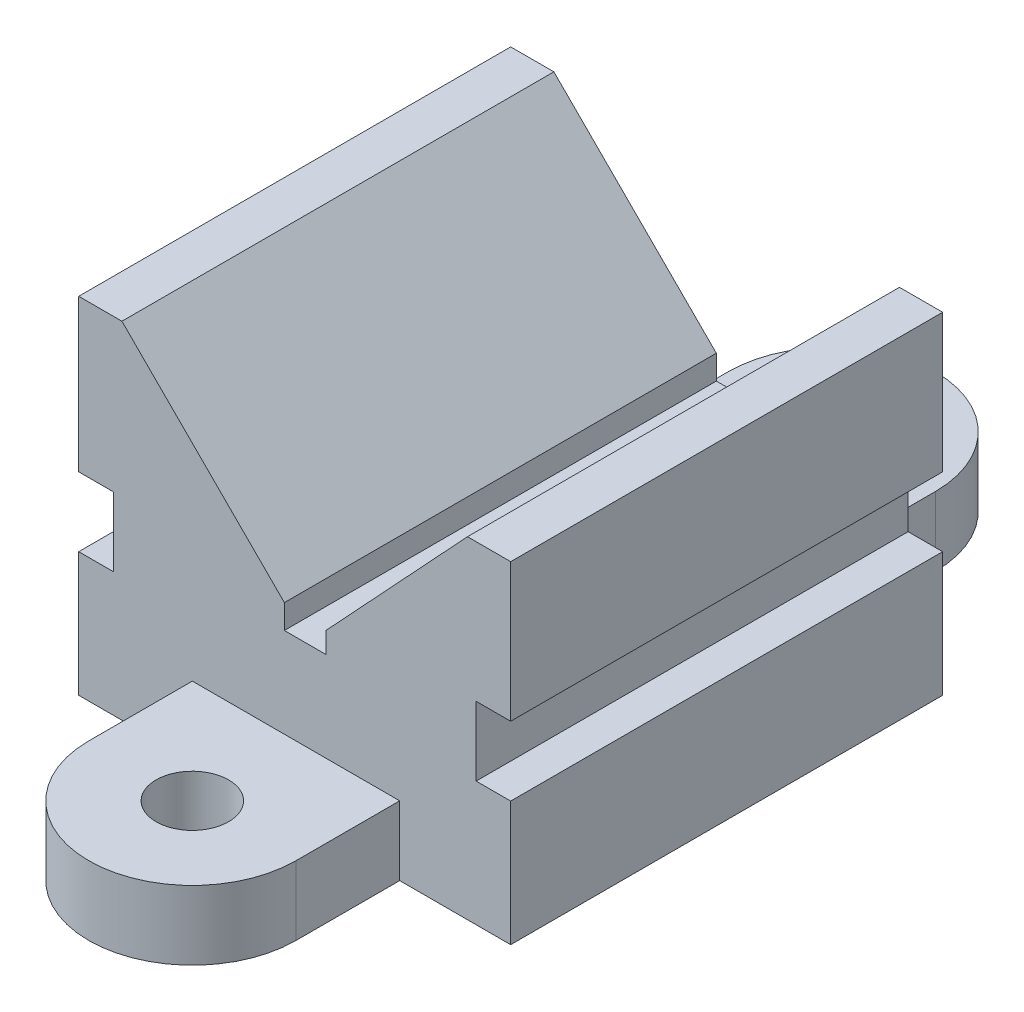
ISO-10303-21;
HEADER;
FILE_DESCRIPTION(('STEP AP214'),'2;1');
FILE_NAME('part.step','',(''),(''),'','','');
FILE_SCHEMA(('AUTOMOTIVE_DESIGN { 1 0 10303 214 1 1 1 1 }'));
ENDSEC;
DATA;
#1=APPLICATION_CONTEXT('core data for automotive mechanical design processes');
#2=APPLICATION_PROTOCOL_DEFINITION('international standard','automotive_design',2000,#1);
#3=PRODUCT_CONTEXT('',#1,'mechanical');
#4=PRODUCT('Part','Part','',(#3));
#5=PRODUCT_RELATED_PRODUCT_CATEGORY('part','',(#4));
#6=PRODUCT_DEFINITION_FORMATION('','',#4);
#7=PRODUCT_DEFINITION_CONTEXT('part definition',#1,'design');
#8=PRODUCT_DEFINITION('design','',#6,#7);
#9=PRODUCT_DEFINITION_SHAPE('','',#8);
#10=(LENGTH_UNIT() NAMED_UNIT(*) SI_UNIT(.MILLI.,.METRE.));
#11=(NAMED_UNIT(*) PLANE_ANGLE_UNIT() SI_UNIT($,.RADIAN.));
#12=(NAMED_UNIT(*) SI_UNIT($,.STERADIAN.) SOLID_ANGLE_UNIT());
#13=UNCERTAINTY_MEASURE_WITH_UNIT(LENGTH_MEASURE(1.E-05),#10,'distance_accuracy_value','');
#14=(GEOMETRIC_REPRESENTATION_CONTEXT(3) GLOBAL_UNCERTAINTY_ASSIGNED_CONTEXT((#13)) GLOBAL_UNIT_ASSIGNED_CONTEXT((#10,
#11,#12)) REPRESENTATION_CONTEXT('',''));
#15=CARTESIAN_POINT('',(0.,0.,0.));
#16=DIRECTION('',(0.,0.,1.));
#17=DIRECTION('',(1.,0.,0.));
#18=AXIS2_PLACEMENT_3D('',#15,#16,#17);
#19=CARTESIAN_POINT('',(-40.4580152671756,36.,125.));
#20=DIRECTION('',(1.,0.,0.));
#21=DIRECTION('',(0.,1.,0.));
#22=AXIS2_PLACEMENT_3D('',#19,#20,#21);
#23=PLANE('',#22);
#24=DIRECTION('',(0.,-1.,0.));
#25=VECTOR('',#24,1.);
#26=CARTESIAN_POINT('',(-40.4580152671756,36.,0.));
#27=LINE('',#26,#25);
#28=CARTESIAN_POINT('',(-40.4580152671756,36.,0.));
#29=VERTEX_POINT('',#28);
#30=CARTESIAN_POINT('',(-40.4580152671756,0.,0.));
#31=VERTEX_POINT('',#30);
#32=EDGE_CURVE('E266',#29,#31,#27,.T.);
#33=ORIENTED_EDGE('',*,*,#32,.T.);
#34=DIRECTION('',(0.,0.,-1.));
#35=VECTOR('',#34,1.);
#36=CARTESIAN_POINT('',(-40.4580152671756,0.,125.));
#37=LINE('',#36,#35);
#38=CARTESIAN_POINT('',(-40.4580152671756,0.,125.));
#39=VERTEX_POINT('',#38);
#40=EDGE_CURVE('E393',#39,#31,#37,.T.);
#41=ORIENTED_EDGE('',*,*,#40,.F.);
#42=DIRECTION('',(0.,-1.,0.));
#43=VECTOR('',#42,1.);
#44=CARTESIAN_POINT('',(-40.4580152671756,36.,125.));
#45=LINE('',#44,#43);
#46=CARTESIAN_POINT('',(-40.4580152671756,36.,125.));
#47=VERTEX_POINT('',#46);
#48=EDGE_CURVE('E270',#47,#39,#45,.T.);
#49=ORIENTED_EDGE('',*,*,#48,.F.);
#50=DIRECTION('',(0.,0.,-1.));
#51=VECTOR('',#50,1.);
#52=CARTESIAN_POINT('',(-40.4580152671756,36.,125.));
#53=LINE('',#52,#51);
#54=EDGE_CURVE('E308',#47,#29,#53,.T.);
#55=ORIENTED_EDGE('',*,*,#54,.T.);
#56=EDGE_LOOP('',(#33,#41,#49,#55));
#57=FACE_BOUND('',#56,.T.);
#58=ADVANCED_FACE('F39',(#57),#23,.F.);
#59=CARTESIAN_POINT('',(-40.4580152671756,0.,125.));
#60=DIRECTION('',(0.,1.,0.));
#61=DIRECTION('',(0.,0.,1.));
#62=AXIS2_PLACEMENT_3D('',#59,#60,#61);
#63=PLANE('',#62);
#64=DIRECTION('',(1.,0.,0.));
#65=VECTOR('',#64,1.);
#66=CARTESIAN_POINT('',(-40.4580152671756,0.,0.));
#67=LINE('',#66,#65);
#68=CARTESIAN_POINT('',(-7.57863831219291,0.,0.));
#69=VERTEX_POINT('',#68);
#70=EDGE_CURVE('E309',#31,#69,#67,.T.);
#71=ORIENTED_EDGE('',*,*,#70,.T.);
#72=DIRECTION('',(0.,0.,-1.));
#73=VECTOR('',#72,1.);
#74=CARTESIAN_POINT('',(-7.57863831219292,0.,155.));
#75=LINE('',#74,#73);
#76=CARTESIAN_POINT('',(-7.5786383121929,0.,-30.));
#77=VERTEX_POINT('',#76);
#78=EDGE_CURVE('E253',#69,#77,#75,.T.);
#79=ORIENTED_EDGE('',*,*,#78,.T.);
#80=CARTESIAN_POINT('',(22.4213616878071,0.,-30.));
#81=DIRECTION('',(0.,-1.,0.));
#82=DIRECTION('',(0.,0.,-1.));
#83=AXIS2_PLACEMENT_3D('',#80,#81,#82);
#84=CIRCLE('',#83,30.);
#85=CARTESIAN_POINT('',(52.4213616878071,0.,-30.));
#86=VERTEX_POINT('',#85);
#87=EDGE_CURVE('E255',#77,#86,#84,.T.);
#88=ORIENTED_EDGE('',*,*,#87,.T.);
#89=DIRECTION('',(0.,0.,1.));
#90=VECTOR('',#89,1.);
#91=CARTESIAN_POINT('',(52.4213616878071,0.,155.));
#92=LINE('',#91,#90);
#93=CARTESIAN_POINT('',(52.4213616878071,0.,0.));
#94=VERTEX_POINT('',#93);
#95=EDGE_CURVE('E237',#86,#94,#92,.T.);
#96=ORIENTED_EDGE('',*,*,#95,.T.);
#97=CARTESIAN_POINT('',(84.5419847328244,0.,0.));
#98=VERTEX_POINT('',#97);
#99=EDGE_CURVE('E310',#94,#98,#67,.T.);
#100=ORIENTED_EDGE('',*,*,#99,.T.);
#101=DIRECTION('',(0.,0.,-1.));
#102=VECTOR('',#101,1.);
#103=CARTESIAN_POINT('',(84.5419847328244,0.,125.));
#104=LINE('',#103,#102);
#105=CARTESIAN_POINT('',(84.5419847328244,0.,125.));
#106=VERTEX_POINT('',#105);
#107=EDGE_CURVE('E391',#106,#98,#104,.T.);
#108=ORIENTED_EDGE('',*,*,#107,.F.);
#109=DIRECTION('',(1.,0.,0.));
#110=VECTOR('',#109,1.);
#111=CARTESIAN_POINT('',(-40.4580152671756,0.,125.));
#112=LINE('',#111,#110);
#113=CARTESIAN_POINT('',(52.4213616878071,0.,125.));
#114=VERTEX_POINT('',#113);
#115=EDGE_CURVE('E269',#114,#106,#112,.T.);
#116=ORIENTED_EDGE('',*,*,#115,.F.);
#117=CARTESIAN_POINT('',(52.4213616878071,0.,155.));
#118=VERTEX_POINT('',#117);
#119=EDGE_CURVE('E236',#114,#118,#92,.T.);
#120=ORIENTED_EDGE('',*,*,#119,.T.);
#121=CARTESIAN_POINT('',(22.4213616878071,0.,155.));
#122=DIRECTION('',(0.,-1.,0.));
#123=DIRECTION('',(0.,0.,-1.));
#124=AXIS2_PLACEMENT_3D('',#121,#122,#123);
#125=CIRCLE('',#124,30.);
#126=CARTESIAN_POINT('',(-7.57863831219292,0.,155.));
#127=VERTEX_POINT('',#126);
#128=EDGE_CURVE('E248',#118,#127,#125,.T.);
#129=ORIENTED_EDGE('',*,*,#128,.T.);
#130=CARTESIAN_POINT('',(-7.57863831219293,0.,125.));
#131=VERTEX_POINT('',#130);
#132=EDGE_CURVE('E214',#127,#131,#75,.T.);
#133=ORIENTED_EDGE('',*,*,#132,.T.);
#134=EDGE_CURVE('E275',#39,#131,#112,.T.);
#135=ORIENTED_EDGE('',*,*,#134,.F.);
#136=ORIENTED_EDGE('',*,*,#40,.T.);
#137=EDGE_LOOP('',(#71,#79,#88,#96,#100,#108,#116,#120,#129,#133,#135,#136));
#138=FACE_BOUND('',#137,.T.);
#139=CARTESIAN_POINT('',(22.4213616878071,0.,-30.));
#140=DIRECTION('',(0.,-1.,0.));
#141=DIRECTION('',(0.,0.,-1.));
#142=AXIS2_PLACEMENT_3D('',#139,#140,#141);
#143=CIRCLE('',#142,10.5);
#144=CARTESIAN_POINT('',(22.4213616878071,0.,-40.5));
#145=VERTEX_POINT('',#144);
#146=EDGE_CURVE('E241',#145,#145,#143,.T.);
#147=ORIENTED_EDGE('',*,*,#146,.F.);
#148=EDGE_LOOP('',(#147));
#149=FACE_BOUND('',#148,.T.);
#150=CARTESIAN_POINT('',(22.4213616878071,0.,155.));
#151=DIRECTION('',(0.,-1.,0.));
#152=DIRECTION('',(0.,0.,-1.));
#153=AXIS2_PLACEMENT_3D('',#150,#151,#152);
#154=CIRCLE('',#153,10.5);
#155=CARTESIAN_POINT('',(22.4213616878071,0.,144.5));
#156=VERTEX_POINT('',#155);
#157=EDGE_CURVE('E587',#156,#156,#154,.T.);
#158=ORIENTED_EDGE('',*,*,#157,.F.);
#159=EDGE_LOOP('',(#158));
#160=FACE_BOUND('',#159,.T.);
#161=ADVANCED_FACE('F410',(#138,#149,#160),#63,.F.);
#162=CARTESIAN_POINT('',(84.5419847328244,0.,125.));
#163=DIRECTION('',(-1.,0.,0.));
#164=DIRECTION('',(0.,-1.,0.));
#165=AXIS2_PLACEMENT_3D('',#162,#163,#164);
#166=PLANE('',#165);
#167=DIRECTION('',(0.,1.,0.));
#168=VECTOR('',#167,1.);
#169=CARTESIAN_POINT('',(84.5419847328244,0.,0.));
#170=LINE('',#169,#168);
#171=CARTESIAN_POINT('',(84.5419847328244,36.,0.));
#172=VERTEX_POINT('',#171);
#173=EDGE_CURVE('E311',#98,#172,#170,.T.);
#174=ORIENTED_EDGE('',*,*,#173,.T.);
#175=DIRECTION('',(0.,0.,-1.));
#176=VECTOR('',#175,1.);
#177=CARTESIAN_POINT('',(84.5419847328244,36.,125.));
#178=LINE('',#177,#176);
#179=CARTESIAN_POINT('',(84.5419847328244,36.,125.));
#180=VERTEX_POINT('',#179);
#181=EDGE_CURVE('E389',#180,#172,#178,.T.);
#182=ORIENTED_EDGE('',*,*,#181,.F.);
#183=DIRECTION('',(0.,1.,0.));
#184=VECTOR('',#183,1.);
#185=CARTESIAN_POINT('',(84.5419847328244,0.,125.));
#186=LINE('',#185,#184);
#187=EDGE_CURVE('E273',#106,#180,#186,.T.);
#188=ORIENTED_EDGE('',*,*,#187,.F.);
#189=ORIENTED_EDGE('',*,*,#107,.T.);
#190=EDGE_LOOP('',(#174,#182,#188,#189));
#191=FACE_BOUND('',#190,.T.);
#192=ADVANCED_FACE('F489',(#191),#166,.F.);
#193=CARTESIAN_POINT('',(84.5419847328244,36.,125.));
#194=DIRECTION('',(0.,-1.,0.));
#195=DIRECTION('',(1.,0.,0.));
#196=AXIS2_PLACEMENT_3D('',#193,#194,#195);
#197=PLANE('',#196);
#198=DIRECTION('',(-1.,0.,0.));
#199=VECTOR('',#198,1.);
#200=CARTESIAN_POINT('',(84.5419847328244,36.,0.));
#201=LINE('',#200,#199);
#202=CARTESIAN_POINT('',(74.5419847328244,36.,0.));
#203=VERTEX_POINT('',#202);
#204=EDGE_CURVE('E312',#172,#203,#201,.T.);
#205=ORIENTED_EDGE('',*,*,#204,.T.);
#206=DIRECTION('',(0.,0.,-1.));
#207=VECTOR('',#206,1.);
#208=CARTESIAN_POINT('',(74.5419847328244,36.,125.));
#209=LINE('',#208,#207);
#210=CARTESIAN_POINT('',(74.5419847328244,36.,125.));
#211=VERTEX_POINT('',#210);
#212=EDGE_CURVE('E384',#211,#203,#209,.T.);
#213=ORIENTED_EDGE('',*,*,#212,.F.);
#214=DIRECTION('',(-1.,0.,0.));
#215=VECTOR('',#214,1.);
#216=CARTESIAN_POINT('',(84.5419847328244,36.,125.));
#217=LINE('',#216,#215);
#218=EDGE_CURVE('E277',#180,#211,#217,.T.);
#219=ORIENTED_EDGE('',*,*,#218,.F.);
#220=ORIENTED_EDGE('',*,*,#181,.T.);
#221=EDGE_LOOP('',(#205,#213,#219,#220));
#222=FACE_BOUND('',#221,.T.);
#223=ADVANCED_FACE('F486',(#222),#197,.F.);
#224=CARTESIAN_POINT('',(74.5419847328244,36.,125.));
#225=DIRECTION('',(-1.,0.,0.));
#226=DIRECTION('',(0.,0.,1.));
#227=AXIS2_PLACEMENT_3D('',#224,#225,#226);
#228=PLANE('',#227);
#229=DIRECTION('',(0.,1.,0.));
#230=VECTOR('',#229,1.);
#231=CARTESIAN_POINT('',(74.5419847328244,36.,0.));
#232=LINE('',#231,#230);
#233=CARTESIAN_POINT('',(74.5419847328244,56.,0.));
#234=VERTEX_POINT('',#233);
#235=EDGE_CURVE('E320',#203,#234,#232,.T.);
#236=ORIENTED_EDGE('',*,*,#235,.T.);
#237=DIRECTION('',(0.,0.,-1.));
#238=VECTOR('',#237,1.);
#239=CARTESIAN_POINT('',(74.5419847328244,56.,125.));
#240=LINE('',#239,#238);
#241=CARTESIAN_POINT('',(74.5419847328244,56.,125.));
#242=VERTEX_POINT('',#241);
#243=EDGE_CURVE('E385',#242,#234,#240,.T.);
#244=ORIENTED_EDGE('',*,*,#243,.F.);
#245=DIRECTION('',(0.,1.,0.));
#246=VECTOR('',#245,1.);
#247=CARTESIAN_POINT('',(74.5419847328244,36.,125.));
#248=LINE('',#247,#246);
#249=EDGE_CURVE('E279',#211,#242,#248,.T.);
#250=ORIENTED_EDGE('',*,*,#249,.F.);
#251=ORIENTED_EDGE('',*,*,#212,.T.);
#252=EDGE_LOOP('',(#236,#244,#250,#251));
#253=FACE_BOUND('',#252,.T.);
#254=ADVANCED_FACE('F485',(#253),#228,.F.);
#255=CARTESIAN_POINT('',(74.5419847328244,56.,125.));
#256=DIRECTION('',(0.,1.,0.));
#257=DIRECTION('',(0.,0.,1.));
#258=AXIS2_PLACEMENT_3D('',#255,#256,#257);
#259=PLANE('',#258);
#260=DIRECTION('',(1.,0.,0.));
#261=VECTOR('',#260,1.);
#262=CARTESIAN_POINT('',(74.5419847328244,56.,0.));
#263=LINE('',#262,#261);
#264=CARTESIAN_POINT('',(84.5419847328244,56.,0.));
#265=VERTEX_POINT('',#264);
#266=EDGE_CURVE('E317',#234,#265,#263,.T.);
#267=ORIENTED_EDGE('',*,*,#266,.T.);
#268=DIRECTION('',(0.,0.,-1.));
#269=VECTOR('',#268,1.);
#270=CARTESIAN_POINT('',(84.5419847328244,56.,125.));
#271=LINE('',#270,#269);
#272=CARTESIAN_POINT('',(84.5419847328244,56.,125.));
#273=VERTEX_POINT('',#272);
#274=EDGE_CURVE('E377',#273,#265,#271,.T.);
#275=ORIENTED_EDGE('',*,*,#274,.F.);
#276=DIRECTION('',(1.,0.,0.));
#277=VECTOR('',#276,1.);
#278=CARTESIAN_POINT('',(74.5419847328244,56.,125.));
#279=LINE('',#278,#277);
#280=EDGE_CURVE('E278',#242,#273,#279,.T.);
#281=ORIENTED_EDGE('',*,*,#280,.F.);
#282=ORIENTED_EDGE('',*,*,#243,.T.);
#283=EDGE_LOOP('',(#267,#275,#281,#282));
#284=FACE_BOUND('',#283,.T.);
#285=ADVANCED_FACE('F480',(#284),#259,.F.);
#286=CARTESIAN_POINT('',(84.5419847328244,56.,125.));
#287=DIRECTION('',(-1.,0.,0.));
#288=DIRECTION('',(0.,0.,1.));
#289=AXIS2_PLACEMENT_3D('',#286,#287,#288);
#290=PLANE('',#289);
#291=DIRECTION('',(0.,1.,0.));
#292=VECTOR('',#291,1.);
#293=CARTESIAN_POINT('',(84.5419847328244,56.,0.));
#294=LINE('',#293,#292);
#295=CARTESIAN_POINT('',(84.5419847328244,96.,0.));
#296=VERTEX_POINT('',#295);
#297=EDGE_CURVE('E321',#265,#296,#294,.T.);
#298=ORIENTED_EDGE('',*,*,#297,.T.);
#299=DIRECTION('',(0.,0.,-1.));
#300=VECTOR('',#299,1.);
#301=CARTESIAN_POINT('',(84.5419847328244,96.,125.));
#302=LINE('',#301,#300);
#303=CARTESIAN_POINT('',(84.5419847328244,96.,125.));
#304=VERTEX_POINT('',#303);
#305=EDGE_CURVE('E376',#304,#296,#302,.T.);
#306=ORIENTED_EDGE('',*,*,#305,.F.);
#307=DIRECTION('',(0.,1.,0.));
#308=VECTOR('',#307,1.);
#309=CARTESIAN_POINT('',(84.5419847328244,56.,125.));
#310=LINE('',#309,#308);
#311=EDGE_CURVE('E285',#273,#304,#310,.T.);
#312=ORIENTED_EDGE('',*,*,#311,.F.);
#313=ORIENTED_EDGE('',*,*,#274,.T.);
#314=EDGE_LOOP('',(#298,#306,#312,#313));
#315=FACE_BOUND('',#314,.T.);
#316=ADVANCED_FACE('F473',(#315),#290,.F.);
#317=CARTESIAN_POINT('',(84.5419847328244,96.,125.));
#318=DIRECTION('',(0.,-1.,0.));
#319=DIRECTION('',(0.,0.,-1.));
#320=AXIS2_PLACEMENT_3D('',#317,#318,#319);
#321=PLANE('',#320);
#322=DIRECTION('',(-1.,0.,0.));
#323=VECTOR('',#322,1.);
#324=CARTESIAN_POINT('',(84.5419847328244,96.,0.));
#325=LINE('',#324,#323);
#326=CARTESIAN_POINT('',(72.0419847328244,96.,0.));
#327=VERTEX_POINT('',#326);
#328=EDGE_CURVE('E323',#296,#327,#325,.T.);
#329=ORIENTED_EDGE('',*,*,#328,.T.);
#330=DIRECTION('',(0.,0.,-1.));
#331=VECTOR('',#330,1.);
#332=CARTESIAN_POINT('',(72.0419847328244,96.,125.));
#333=LINE('',#332,#331);
#334=CARTESIAN_POINT('',(72.0419847328244,96.,125.));
#335=VERTEX_POINT('',#334);
#336=EDGE_CURVE('E373',#335,#327,#333,.T.);
#337=ORIENTED_EDGE('',*,*,#336,.F.);
#338=DIRECTION('',(-1.,0.,0.));
#339=VECTOR('',#338,1.);
#340=CARTESIAN_POINT('',(84.5419847328244,96.,125.));
#341=LINE('',#340,#339);
#342=EDGE_CURVE('E283',#304,#335,#341,.T.);
#343=ORIENTED_EDGE('',*,*,#342,.F.);
#344=ORIENTED_EDGE('',*,*,#305,.T.);
#345=EDGE_LOOP('',(#329,#337,#343,#344));
#346=FACE_BOUND('',#345,.T.);
#347=ADVANCED_FACE('F470',(#346),#321,.F.);
#348=CARTESIAN_POINT('',(72.0419847328244,96.,125.));
#349=DIRECTION('',(0.731695452994903,-0.68163169238716,0.));
#350=DIRECTION('',(0.68163169238716,0.731695452994903,0.));
#351=AXIS2_PLACEMENT_3D('',#348,#349,#350);
#352=PLANE('',#351);
#353=DIRECTION('',(-0.68163169238716,-0.731695452994903,0.));
#354=VECTOR('',#353,1.);
#355=CARTESIAN_POINT('',(72.0419847328244,96.,0.));
#356=LINE('',#355,#354);
#357=CARTESIAN_POINT('',(31.052534351145,52.,0.));
#358=VERTEX_POINT('',#357);
#359=EDGE_CURVE('E324',#327,#358,#356,.T.);
#360=ORIENTED_EDGE('',*,*,#359,.T.);
#361=DIRECTION('',(0.,0.,-1.));
#362=VECTOR('',#361,1.);
#363=CARTESIAN_POINT('',(31.052534351145,52.,125.));
#364=LINE('',#363,#362);
#365=CARTESIAN_POINT('',(31.052534351145,52.,125.));
#366=VERTEX_POINT('',#365);
#367=EDGE_CURVE('E367',#366,#358,#364,.T.);
#368=ORIENTED_EDGE('',*,*,#367,.F.);
#369=DIRECTION('',(-0.68163169238716,-0.731695452994903,0.));
#370=VECTOR('',#369,1.);
#371=CARTESIAN_POINT('',(72.0419847328244,96.,125.));
#372=LINE('',#371,#370);
#373=EDGE_CURVE('E286',#335,#366,#372,.T.);
#374=ORIENTED_EDGE('',*,*,#373,.F.);
#375=ORIENTED_EDGE('',*,*,#336,.T.);
#376=EDGE_LOOP('',(#360,#368,#374,#375));
#377=FACE_BOUND('',#376,.T.);
#378=ADVANCED_FACE('F465',(#377),#352,.F.);
#379=CARTESIAN_POINT('',(31.052534351145,52.,125.));
#380=DIRECTION('',(1.,0.,0.));
#381=DIRECTION('',(0.,1.,0.));
#382=AXIS2_PLACEMENT_3D('',#379,#380,#381);
#383=PLANE('',#382);
#384=DIRECTION('',(0.,-1.,0.));
#385=VECTOR('',#384,1.);
#386=CARTESIAN_POINT('',(31.052534351145,52.,0.));
#387=LINE('',#386,#385);
#388=CARTESIAN_POINT('',(31.052534351145,46.,0.));
#389=VERTEX_POINT('',#388);
#390=EDGE_CURVE('E330',#358,#389,#387,.T.);
#391=ORIENTED_EDGE('',*,*,#390,.T.);
#392=DIRECTION('',(0.,0.,-1.));
#393=VECTOR('',#392,1.);
#394=CARTESIAN_POINT('',(31.052534351145,46.,125.));
#395=LINE('',#394,#393);
#396=CARTESIAN_POINT('',(31.052534351145,46.,125.));
#397=VERTEX_POINT('',#396);
#398=EDGE_CURVE('E370',#397,#389,#395,.T.);
#399=ORIENTED_EDGE('',*,*,#398,.F.);
#400=DIRECTION('',(0.,-1.,0.));
#401=VECTOR('',#400,1.);
#402=CARTESIAN_POINT('',(31.052534351145,52.,125.));
#403=LINE('',#402,#401);
#404=EDGE_CURVE('E287',#366,#397,#403,.T.);
#405=ORIENTED_EDGE('',*,*,#404,.F.);
#406=ORIENTED_EDGE('',*,*,#367,.T.);
#407=EDGE_LOOP('',(#391,#399,#405,#406));
#408=FACE_BOUND('',#407,.T.);
#409=ADVANCED_FACE('F457',(#408),#383,.F.);
#410=CARTESIAN_POINT('',(31.052534351145,46.,125.));
#411=DIRECTION('',(0.,-1.,0.));
#412=DIRECTION('',(1.,0.,0.));
#413=AXIS2_PLACEMENT_3D('',#410,#411,#412);
#414=PLANE('',#413);
#415=DIRECTION('',(-1.,0.,0.));
#416=VECTOR('',#415,1.);
#417=CARTESIAN_POINT('',(31.052534351145,46.,0.));
#418=LINE('',#417,#416);
#419=CARTESIAN_POINT('',(19.052534351145,46.,0.));
#420=VERTEX_POINT('',#419);
#421=EDGE_CURVE('E328',#389,#420,#418,.T.);
#422=ORIENTED_EDGE('',*,*,#421,.T.);
#423=DIRECTION('',(0.,0.,-1.));
#424=VECTOR('',#423,1.);
#425=CARTESIAN_POINT('',(19.052534351145,46.,125.));
#426=LINE('',#425,#424);
#427=CARTESIAN_POINT('',(19.052534351145,46.,125.));
#428=VERTEX_POINT('',#427);
#429=EDGE_CURVE('E365',#428,#420,#426,.T.);
#430=ORIENTED_EDGE('',*,*,#429,.F.);
#431=DIRECTION('',(-1.,0.,0.));
#432=VECTOR('',#431,1.);
#433=CARTESIAN_POINT('',(31.052534351145,46.,125.));
#434=LINE('',#433,#432);
#435=EDGE_CURVE('E289',#397,#428,#434,.T.);
#436=ORIENTED_EDGE('',*,*,#435,.F.);
#437=ORIENTED_EDGE('',*,*,#398,.T.);
#438=EDGE_LOOP('',(#422,#430,#436,#437));
#439=FACE_BOUND('',#438,.T.);
#440=ADVANCED_FACE('F455',(#439),#414,.F.);
#441=CARTESIAN_POINT('',(19.052534351145,46.,125.));
#442=DIRECTION('',(-1.,0.,0.));
#443=DIRECTION('',(0.,-1.,0.));
#444=AXIS2_PLACEMENT_3D('',#441,#442,#443);
#445=PLANE('',#444);
#446=DIRECTION('',(0.,1.,0.));
#447=VECTOR('',#446,1.);
#448=CARTESIAN_POINT('',(19.052534351145,46.,0.));
#449=LINE('',#448,#447);
#450=CARTESIAN_POINT('',(19.052534351145,52.9894503816794,0.));
#451=VERTEX_POINT('',#450);
#452=EDGE_CURVE('E332',#420,#451,#449,.T.);
#453=ORIENTED_EDGE('',*,*,#452,.T.);
#454=DIRECTION('',(0.,0.,-1.));
#455=VECTOR('',#454,1.);
#456=CARTESIAN_POINT('',(19.052534351145,52.9894503816794,125.));
#457=LINE('',#456,#455);
#458=CARTESIAN_POINT('',(19.052534351145,52.9894503816794,125.));
#459=VERTEX_POINT('',#458);
#460=EDGE_CURVE('E363',#459,#451,#457,.T.);
#461=ORIENTED_EDGE('',*,*,#460,.F.);
#462=DIRECTION('',(0.,1.,0.));
#463=VECTOR('',#462,1.);
#464=CARTESIAN_POINT('',(19.052534351145,46.,125.));
#465=LINE('',#464,#463);
#466=EDGE_CURVE('E295',#428,#459,#465,.T.);
#467=ORIENTED_EDGE('',*,*,#466,.F.);
#468=ORIENTED_EDGE('',*,*,#429,.T.);
#469=EDGE_LOOP('',(#453,#461,#467,#468));
#470=FACE_BOUND('',#469,.T.);
#471=ADVANCED_FACE('F450',(#470),#445,.F.);
#472=CARTESIAN_POINT('',(19.052534351145,52.9894503816794,125.));
#473=DIRECTION('',(-0.707106781186547,-0.707106781186548,0.));
#474=DIRECTION('',(0.707106781186548,-0.707106781186547,0.));
#475=AXIS2_PLACEMENT_3D('',#472,#473,#474);
#476=PLANE('',#475);
#477=DIRECTION('',(-0.707106781186548,0.707106781186547,0.));
#478=VECTOR('',#477,1.);
#479=CARTESIAN_POINT('',(19.052534351145,52.9894503816794,0.));
#480=LINE('',#479,#478);
#481=CARTESIAN_POINT('',(-27.9580152671756,100.,0.));
#482=VERTEX_POINT('',#481);
#483=EDGE_CURVE('E334',#451,#482,#480,.T.);
#484=ORIENTED_EDGE('',*,*,#483,.T.);
#485=DIRECTION('',(0.,0.,-1.));
#486=VECTOR('',#485,1.);
#487=CARTESIAN_POINT('',(-27.9580152671756,100.,125.));
#488=LINE('',#487,#486);
#489=CARTESIAN_POINT('',(-27.9580152671756,100.,125.));
#490=VERTEX_POINT('',#489);
#491=EDGE_CURVE('E357',#490,#482,#488,.T.);
#492=ORIENTED_EDGE('',*,*,#491,.F.);
#493=DIRECTION('',(-0.707106781186548,0.707106781186547,0.));
#494=VECTOR('',#493,1.);
#495=CARTESIAN_POINT('',(19.052534351145,52.9894503816794,125.));
#496=LINE('',#495,#494);
#497=EDGE_CURVE('E294',#459,#490,#496,.T.);
#498=ORIENTED_EDGE('',*,*,#497,.F.);
#499=ORIENTED_EDGE('',*,*,#460,.T.);
#500=EDGE_LOOP('',(#484,#492,#498,#499));
#501=FACE_BOUND('',#500,.T.);
#502=ADVANCED_FACE('F442',(#501),#476,.F.);
#503=CARTESIAN_POINT('',(-27.9580152671756,100.,125.));
#504=DIRECTION('',(0.,-1.,0.));
#505=DIRECTION('',(0.,0.,-1.));
#506=AXIS2_PLACEMENT_3D('',#503,#504,#505);
#507=PLANE('',#506);
#508=DIRECTION('',(-1.,0.,0.));
#509=VECTOR('',#508,1.);
#510=CARTESIAN_POINT('',(-27.9580152671756,100.,0.));
#511=LINE('',#510,#509);
#512=CARTESIAN_POINT('',(-40.4580152671756,100.,0.));
#513=VERTEX_POINT('',#512);
#514=EDGE_CURVE('E333',#482,#513,#511,.T.);
#515=ORIENTED_EDGE('',*,*,#514,.T.);
#516=DIRECTION('',(0.,0.,-1.));
#517=VECTOR('',#516,1.);
#518=CARTESIAN_POINT('',(-40.4580152671756,100.,125.));
#519=LINE('',#518,#517);
#520=CARTESIAN_POINT('',(-40.4580152671756,100.,125.));
#521=VERTEX_POINT('',#520);
#522=EDGE_CURVE('E354',#521,#513,#519,.T.);
#523=ORIENTED_EDGE('',*,*,#522,.F.);
#524=DIRECTION('',(-1.,0.,0.));
#525=VECTOR('',#524,1.);
#526=CARTESIAN_POINT('',(-27.9580152671756,100.,125.));
#527=LINE('',#526,#525);
#528=EDGE_CURVE('E296',#490,#521,#527,.T.);
#529=ORIENTED_EDGE('',*,*,#528,.F.);
#530=ORIENTED_EDGE('',*,*,#491,.T.);
#531=EDGE_LOOP('',(#515,#523,#529,#530));
#532=FACE_BOUND('',#531,.T.);
#533=ADVANCED_FACE('F440',(#532),#507,.F.);
#534=CARTESIAN_POINT('',(-40.4580152671756,100.,125.));
#535=DIRECTION('',(1.,0.,0.));
#536=DIRECTION('',(0.,1.,0.));
#537=AXIS2_PLACEMENT_3D('',#534,#535,#536);
#538=PLANE('',#537);
#539=DIRECTION('',(0.,-1.,0.));
#540=VECTOR('',#539,1.);
#541=CARTESIAN_POINT('',(-40.4580152671756,100.,0.));
#542=LINE('',#541,#540);
#543=CARTESIAN_POINT('',(-40.4580152671756,56.,0.));
#544=VERTEX_POINT('',#543);
#545=EDGE_CURVE('E340',#513,#544,#542,.T.);
#546=ORIENTED_EDGE('',*,*,#545,.T.);
#547=DIRECTION('',(0.,0.,-1.));
#548=VECTOR('',#547,1.);
#549=CARTESIAN_POINT('',(-40.4580152671756,56.,125.));
#550=LINE('',#549,#548);
#551=CARTESIAN_POINT('',(-40.4580152671756,56.,125.));
#552=VERTEX_POINT('',#551);
#553=EDGE_CURVE('E355',#552,#544,#550,.T.);
#554=ORIENTED_EDGE('',*,*,#553,.F.);
#555=DIRECTION('',(0.,-1.,0.));
#556=VECTOR('',#555,1.);
#557=CARTESIAN_POINT('',(-40.4580152671756,100.,125.));
#558=LINE('',#557,#556);
#559=EDGE_CURVE('E297',#521,#552,#558,.T.);
#560=ORIENTED_EDGE('',*,*,#559,.F.);
#561=ORIENTED_EDGE('',*,*,#522,.T.);
#562=EDGE_LOOP('',(#546,#554,#560,#561));
#563=FACE_BOUND('',#562,.T.);
#564=ADVANCED_FACE('F435',(#563),#538,.F.);
#565=CARTESIAN_POINT('',(-40.4580152671756,56.,125.));
#566=DIRECTION('',(0.,1.,0.));
#567=DIRECTION('',(0.,0.,1.));
#568=AXIS2_PLACEMENT_3D('',#565,#566,#567);
#569=PLANE('',#568);
#570=DIRECTION('',(1.,0.,0.));
#571=VECTOR('',#570,1.);
#572=CARTESIAN_POINT('',(-40.4580152671756,56.,0.));
#573=LINE('',#572,#571);
#574=CARTESIAN_POINT('',(-30.4580152671756,56.,0.));
#575=VERTEX_POINT('',#574);
#576=EDGE_CURVE('E338',#544,#575,#573,.T.);
#577=ORIENTED_EDGE('',*,*,#576,.T.);
#578=DIRECTION('',(0.,0.,-1.));
#579=VECTOR('',#578,1.);
#580=CARTESIAN_POINT('',(-30.4580152671756,56.,125.));
#581=LINE('',#580,#579);
#582=CARTESIAN_POINT('',(-30.4580152671756,56.,125.));
#583=VERTEX_POINT('',#582);
#584=EDGE_CURVE('E349',#583,#575,#581,.T.);
#585=ORIENTED_EDGE('',*,*,#584,.F.);
#586=DIRECTION('',(1.,0.,0.));
#587=VECTOR('',#586,1.);
#588=CARTESIAN_POINT('',(-40.4580152671756,56.,125.));
#589=LINE('',#588,#587);
#590=EDGE_CURVE('E299',#552,#583,#589,.T.);
#591=ORIENTED_EDGE('',*,*,#590,.F.);
#592=ORIENTED_EDGE('',*,*,#553,.T.);
#593=EDGE_LOOP('',(#577,#585,#591,#592));
#594=FACE_BOUND('',#593,.T.);
#595=ADVANCED_FACE('F426',(#594),#569,.F.);
#596=CARTESIAN_POINT('',(-30.4580152671756,56.,125.));
#597=DIRECTION('',(1.,0.,0.));
#598=DIRECTION('',(0.,1.,0.));
#599=AXIS2_PLACEMENT_3D('',#596,#597,#598);
#600=PLANE('',#599);
#601=DIRECTION('',(0.,-1.,0.));
#602=VECTOR('',#601,1.);
#603=CARTESIAN_POINT('',(-30.4580152671756,56.,0.));
#604=LINE('',#603,#602);
#605=CARTESIAN_POINT('',(-30.4580152671756,36.,0.));
#606=VERTEX_POINT('',#605);
#607=EDGE_CURVE('E341',#575,#606,#604,.T.);
#608=ORIENTED_EDGE('',*,*,#607,.T.);
#609=DIRECTION('',(0.,0.,-1.));
#610=VECTOR('',#609,1.);
#611=CARTESIAN_POINT('',(-30.4580152671756,36.,125.));
#612=LINE('',#611,#610);
#613=CARTESIAN_POINT('',(-30.4580152671756,36.,125.));
#614=VERTEX_POINT('',#613);
#615=EDGE_CURVE('E347',#614,#606,#612,.T.);
#616=ORIENTED_EDGE('',*,*,#615,.F.);
#617=DIRECTION('',(0.,-1.,0.));
#618=VECTOR('',#617,1.);
#619=CARTESIAN_POINT('',(-30.4580152671756,56.,125.));
#620=LINE('',#619,#618);
#621=EDGE_CURVE('E305',#583,#614,#620,.T.);
#622=ORIENTED_EDGE('',*,*,#621,.F.);
#623=ORIENTED_EDGE('',*,*,#584,.T.);
#624=EDGE_LOOP('',(#608,#616,#622,#623));
#625=FACE_BOUND('',#624,.T.);
#626=ADVANCED_FACE('F425',(#625),#600,.F.);
#627=CARTESIAN_POINT('',(-30.4580152671756,36.,125.));
#628=DIRECTION('',(0.,-1.,0.));
#629=DIRECTION('',(0.,0.,-1.));
#630=AXIS2_PLACEMENT_3D('',#627,#628,#629);
#631=PLANE('',#630);
#632=DIRECTION('',(-1.,0.,0.));
#633=VECTOR('',#632,1.);
#634=CARTESIAN_POINT('',(-30.4580152671756,36.,0.));
#635=LINE('',#634,#633);
#636=EDGE_CURVE('E271',#606,#29,#635,.T.);
#637=ORIENTED_EDGE('',*,*,#636,.T.);
#638=ORIENTED_EDGE('',*,*,#54,.F.);
#639=DIRECTION('',(-1.,0.,0.));
#640=VECTOR('',#639,1.);
#641=CARTESIAN_POINT('',(-30.4580152671756,36.,125.));
#642=LINE('',#641,#640);
#643=EDGE_CURVE('E303',#614,#47,#642,.T.);
#644=ORIENTED_EDGE('',*,*,#643,.F.);
#645=ORIENTED_EDGE('',*,*,#615,.T.);
#646=EDGE_LOOP('',(#637,#638,#644,#645));
#647=FACE_BOUND('',#646,.T.);
#648=ADVANCED_FACE('F417',(#647),#631,.F.);
#649=CARTESIAN_POINT('',(0.,0.,125.));
#650=DIRECTION('',(0.,0.,1.));
#651=DIRECTION('',(1.,0.,0.));
#652=AXIS2_PLACEMENT_3D('',#649,#650,#651);
#653=PLANE('',#652);
#654=DIRECTION('',(0.,1.,0.));
#655=VECTOR('',#654,1.);
#656=CARTESIAN_POINT('',(52.4213616878071,0.,125.));
#657=LINE('',#656,#655);
#658=CARTESIAN_POINT('',(52.4213616878071,20.,125.));
#659=VERTEX_POINT('',#658);
#660=EDGE_CURVE('E262',#114,#659,#657,.T.);
#661=ORIENTED_EDGE('',*,*,#660,.F.);
#662=ORIENTED_EDGE('',*,*,#115,.T.);
#663=ORIENTED_EDGE('',*,*,#187,.T.);
#664=ORIENTED_EDGE('',*,*,#218,.T.);
#665=ORIENTED_EDGE('',*,*,#249,.T.);
#666=ORIENTED_EDGE('',*,*,#280,.T.);
#667=ORIENTED_EDGE('',*,*,#311,.T.);
#668=ORIENTED_EDGE('',*,*,#342,.T.);
#669=ORIENTED_EDGE('',*,*,#373,.T.);
#670=ORIENTED_EDGE('',*,*,#404,.T.);
#671=ORIENTED_EDGE('',*,*,#435,.T.);
#672=ORIENTED_EDGE('',*,*,#466,.T.);
#673=ORIENTED_EDGE('',*,*,#497,.T.);
#674=ORIENTED_EDGE('',*,*,#528,.T.);
#675=ORIENTED_EDGE('',*,*,#559,.T.);
#676=ORIENTED_EDGE('',*,*,#590,.T.);
#677=ORIENTED_EDGE('',*,*,#621,.T.);
#678=ORIENTED_EDGE('',*,*,#643,.T.);
#679=ORIENTED_EDGE('',*,*,#48,.T.);
#680=ORIENTED_EDGE('',*,*,#134,.T.);
#681=DIRECTION('',(0.,-1.,0.));
#682=VECTOR('',#681,1.);
#683=CARTESIAN_POINT('',(-7.57863831219292,0.,125.));
#684=LINE('',#683,#682);
#685=CARTESIAN_POINT('',(-7.57863831219293,20.,125.));
#686=VERTEX_POINT('',#685);
#687=EDGE_CURVE('E59',#686,#131,#684,.T.);
#688=ORIENTED_EDGE('',*,*,#687,.F.);
#689=DIRECTION('',(1.,0.,0.));
#690=VECTOR('',#689,1.);
#691=CARTESIAN_POINT('',(0.,20.,125.));
#692=LINE('',#691,#690);
#693=EDGE_CURVE('E52',#686,#659,#692,.T.);
#694=ORIENTED_EDGE('',*,*,#693,.T.);
#695=EDGE_LOOP('',(#661,#662,#663,#664,#665,#666,#667,#668,#669,#670,#671,#672,#673,#674,#675,
#676,#677,#678,#679,#680,#688,#694));
#696=FACE_BOUND('',#695,.T.);
#697=ADVANCED_FACE('F513',(#696),#653,.T.);
#698=CARTESIAN_POINT('',(0.,0.,0.));
#699=DIRECTION('',(0.,0.,1.));
#700=DIRECTION('',(1.,0.,0.));
#701=AXIS2_PLACEMENT_3D('',#698,#699,#700);
#702=PLANE('',#701);
#703=ORIENTED_EDGE('',*,*,#99,.F.);
#704=DIRECTION('',(0.,1.,0.));
#705=VECTOR('',#704,1.);
#706=CARTESIAN_POINT('',(52.4213616878071,0.,0.));
#707=LINE('',#706,#705);
#708=CARTESIAN_POINT('',(52.4213616878071,20.,0.));
#709=VERTEX_POINT('',#708);
#710=EDGE_CURVE('E11',#94,#709,#707,.T.);
#711=ORIENTED_EDGE('',*,*,#710,.T.);
#712=DIRECTION('',(1.,0.,0.));
#713=VECTOR('',#712,1.);
#714=CARTESIAN_POINT('',(0.,20.,0.));
#715=LINE('',#714,#713);
#716=CARTESIAN_POINT('',(-7.57863831219291,20.,0.));
#717=VERTEX_POINT('',#716);
#718=EDGE_CURVE('E400',#717,#709,#715,.T.);
#719=ORIENTED_EDGE('',*,*,#718,.F.);
#720=DIRECTION('',(0.,-1.,0.));
#721=VECTOR('',#720,1.);
#722=CARTESIAN_POINT('',(-7.57863831219291,0.,0.));
#723=LINE('',#722,#721);
#724=EDGE_CURVE('E46',#717,#69,#723,.T.);
#725=ORIENTED_EDGE('',*,*,#724,.T.);
#726=ORIENTED_EDGE('',*,*,#70,.F.);
#727=ORIENTED_EDGE('',*,*,#32,.F.);
#728=ORIENTED_EDGE('',*,*,#636,.F.);
#729=ORIENTED_EDGE('',*,*,#607,.F.);
#730=ORIENTED_EDGE('',*,*,#576,.F.);
#731=ORIENTED_EDGE('',*,*,#545,.F.);
#732=ORIENTED_EDGE('',*,*,#514,.F.);
#733=ORIENTED_EDGE('',*,*,#483,.F.);
#734=ORIENTED_EDGE('',*,*,#452,.F.);
#735=ORIENTED_EDGE('',*,*,#421,.F.);
#736=ORIENTED_EDGE('',*,*,#390,.F.);
#737=ORIENTED_EDGE('',*,*,#359,.F.);
#738=ORIENTED_EDGE('',*,*,#328,.F.);
#739=ORIENTED_EDGE('',*,*,#297,.F.);
#740=ORIENTED_EDGE('',*,*,#266,.F.);
#741=ORIENTED_EDGE('',*,*,#235,.F.);
#742=ORIENTED_EDGE('',*,*,#204,.F.);
#743=ORIENTED_EDGE('',*,*,#173,.F.);
#744=EDGE_LOOP('',(#703,#711,#719,#725,#726,#727,#728,#729,#730,#731,#732,#733,#734,#735,#736,
#737,#738,#739,#740,#741,#742,#743));
#745=FACE_BOUND('',#744,.T.);
#746=ADVANCED_FACE('F405',(#745),#702,.F.);
#747=CARTESIAN_POINT('',(22.4213616878071,20.,-30.));
#748=DIRECTION('',(0.,-1.,0.));
#749=DIRECTION('',(0.,0.,-1.));
#750=AXIS2_PLACEMENT_3D('',#747,#748,#749);
#751=CYLINDRICAL_SURFACE('',#750,30.);
#752=ORIENTED_EDGE('',*,*,#87,.F.);
#753=DIRECTION('',(0.,-1.,0.));
#754=VECTOR('',#753,1.);
#755=CARTESIAN_POINT('',(-7.5786383121929,20.,-30.));
#756=LINE('',#755,#754);
#757=CARTESIAN_POINT('',(-7.5786383121929,20.,-30.));
#758=VERTEX_POINT('',#757);
#759=EDGE_CURVE('E219',#758,#77,#756,.T.);
#760=ORIENTED_EDGE('',*,*,#759,.F.);
#761=CARTESIAN_POINT('',(22.4213616878071,20.,-30.));
#762=DIRECTION('',(0.,-1.,0.));
#763=DIRECTION('',(0.,0.,-1.));
#764=AXIS2_PLACEMENT_3D('',#761,#762,#763);
#765=CIRCLE('',#764,30.);
#766=CARTESIAN_POINT('',(52.4213616878071,20.,-30.));
#767=VERTEX_POINT('',#766);
#768=EDGE_CURVE('E228',#758,#767,#765,.T.);
#769=ORIENTED_EDGE('',*,*,#768,.T.);
#770=DIRECTION('',(0.,-1.,0.));
#771=VECTOR('',#770,1.);
#772=CARTESIAN_POINT('',(52.4213616878071,20.,-30.));
#773=LINE('',#772,#771);
#774=EDGE_CURVE('E256',#767,#86,#773,.T.);
#775=ORIENTED_EDGE('',*,*,#774,.T.);
#776=EDGE_LOOP('',(#752,#760,#769,#775));
#777=FACE_BOUND('',#776,.T.);
#778=ADVANCED_FACE('F504',(#777),#751,.T.);
#779=CARTESIAN_POINT('',(22.4213616878071,20.,-30.));
#780=DIRECTION('',(0.,-1.,0.));
#781=DIRECTION('',(0.,0.,-1.));
#782=AXIS2_PLACEMENT_3D('',#779,#780,#781);
#783=CYLINDRICAL_SURFACE('',#782,10.5);
#784=CARTESIAN_POINT('',(22.4213616878071,20.,-30.));
#785=DIRECTION('',(0.,-1.,0.));
#786=DIRECTION('',(0.,0.,-1.));
#787=AXIS2_PLACEMENT_3D('',#784,#785,#786);
#788=CIRCLE('',#787,10.5);
#789=CARTESIAN_POINT('',(22.4213616878071,20.,-40.5));
#790=VERTEX_POINT('',#789);
#791=EDGE_CURVE('E252',#790,#790,#788,.T.);
#792=ORIENTED_EDGE('',*,*,#791,.F.);
#793=EDGE_LOOP('',(#792));
#794=FACE_BOUND('',#793,.T.);
#795=ORIENTED_EDGE('',*,*,#146,.T.);
#796=EDGE_LOOP('',(#795));
#797=FACE_BOUND('',#796,.T.);
#798=ADVANCED_FACE('F510',(#794,#797),#783,.F.);
#799=CARTESIAN_POINT('',(22.4213616878071,20.,155.));
#800=DIRECTION('',(0.,-1.,0.));
#801=DIRECTION('',(0.,0.,-1.));
#802=AXIS2_PLACEMENT_3D('',#799,#800,#801);
#803=PLANE('',#802);
#804=ORIENTED_EDGE('',*,*,#791,.T.);
#805=EDGE_LOOP('',(#804));
#806=FACE_BOUND('',#805,.T.);
#807=DIRECTION('',(0.,0.,-1.));
#808=VECTOR('',#807,1.);
#809=CARTESIAN_POINT('',(-7.57863831219292,20.,155.));
#810=LINE('',#809,#808);
#811=EDGE_CURVE('E229',#717,#758,#810,.T.);
#812=ORIENTED_EDGE('',*,*,#811,.F.);
#813=ORIENTED_EDGE('',*,*,#718,.T.);
#814=DIRECTION('',(0.,0.,1.));
#815=VECTOR('',#814,1.);
#816=CARTESIAN_POINT('',(52.4213616878071,20.,155.));
#817=LINE('',#816,#815);
#818=EDGE_CURVE('E222',#767,#709,#817,.T.);
#819=ORIENTED_EDGE('',*,*,#818,.F.);
#820=ORIENTED_EDGE('',*,*,#768,.F.);
#821=EDGE_LOOP('',(#812,#813,#819,#820));
#822=FACE_BOUND('',#821,.T.);
#823=ADVANCED_FACE('F501',(#806,#822),#803,.F.);
#824=CARTESIAN_POINT('',(-7.57863831219292,20.,155.));
#825=DIRECTION('',(-1.,0.,0.));
#826=DIRECTION('',(0.,0.,1.));
#827=AXIS2_PLACEMENT_3D('',#824,#825,#826);
#828=PLANE('',#827);
#829=ORIENTED_EDGE('',*,*,#724,.F.);
#830=ORIENTED_EDGE('',*,*,#811,.T.);
#831=ORIENTED_EDGE('',*,*,#759,.T.);
#832=ORIENTED_EDGE('',*,*,#78,.F.);
#833=EDGE_LOOP('',(#829,#830,#831,#832));
#834=FACE_BOUND('',#833,.T.);
#835=ADVANCED_FACE('F502',(#834),#828,.T.);
#836=CARTESIAN_POINT('',(52.4213616878071,20.,155.));
#837=DIRECTION('',(1.,0.,0.));
#838=DIRECTION('',(0.,0.,-1.));
#839=AXIS2_PLACEMENT_3D('',#836,#837,#838);
#840=PLANE('',#839);
#841=ORIENTED_EDGE('',*,*,#710,.F.);
#842=ORIENTED_EDGE('',*,*,#95,.F.);
#843=ORIENTED_EDGE('',*,*,#774,.F.);
#844=ORIENTED_EDGE('',*,*,#818,.T.);
#845=EDGE_LOOP('',(#841,#842,#843,#844));
#846=FACE_BOUND('',#845,.T.);
#847=ADVANCED_FACE('F500',(#846),#840,.T.);
#848=CARTESIAN_POINT('',(22.4213616878071,20.,155.));
#849=DIRECTION('',(0.,-1.,0.));
#850=DIRECTION('',(0.,0.,-1.));
#851=AXIS2_PLACEMENT_3D('',#848,#849,#850);
#852=CYLINDRICAL_SURFACE('',#851,30.);
#853=ORIENTED_EDGE('',*,*,#128,.F.);
#854=DIRECTION('',(0.,-1.,0.));
#855=VECTOR('',#854,1.);
#856=CARTESIAN_POINT('',(52.4213616878071,20.,155.));
#857=LINE('',#856,#855);
#858=CARTESIAN_POINT('',(52.4213616878071,20.,155.));
#859=VERTEX_POINT('',#858);
#860=EDGE_CURVE('E234',#859,#118,#857,.T.);
#861=ORIENTED_EDGE('',*,*,#860,.F.);
#862=CARTESIAN_POINT('',(22.4213616878071,20.,155.));
#863=DIRECTION('',(0.,-1.,0.));
#864=DIRECTION('',(0.,0.,-1.));
#865=AXIS2_PLACEMENT_3D('',#862,#863,#864);
#866=CIRCLE('',#865,30.);
#867=CARTESIAN_POINT('',(-7.57863831219292,20.,155.));
#868=VERTEX_POINT('',#867);
#869=EDGE_CURVE('E227',#859,#868,#866,.T.);
#870=ORIENTED_EDGE('',*,*,#869,.T.);
#871=DIRECTION('',(0.,-1.,0.));
#872=VECTOR('',#871,1.);
#873=CARTESIAN_POINT('',(-7.57863831219292,20.,155.));
#874=LINE('',#873,#872);
#875=EDGE_CURVE('E209',#868,#127,#874,.T.);
#876=ORIENTED_EDGE('',*,*,#875,.T.);
#877=EDGE_LOOP('',(#853,#861,#870,#876));
#878=FACE_BOUND('',#877,.T.);
#879=ADVANCED_FACE('F232',(#878),#852,.T.);
#880=ORIENTED_EDGE('',*,*,#119,.F.);
#881=ORIENTED_EDGE('',*,*,#660,.T.);
#882=EDGE_CURVE('E246',#659,#859,#817,.T.);
#883=ORIENTED_EDGE('',*,*,#882,.T.);
#884=ORIENTED_EDGE('',*,*,#860,.T.);
#885=EDGE_LOOP('',(#880,#881,#883,#884));
#886=FACE_BOUND('',#885,.T.);
#887=ADVANCED_FACE('F561',(#886),#840,.T.);
#888=EDGE_CURVE('E213',#868,#686,#810,.T.);
#889=ORIENTED_EDGE('',*,*,#888,.T.);
#890=ORIENTED_EDGE('',*,*,#687,.T.);
#891=ORIENTED_EDGE('',*,*,#132,.F.);
#892=ORIENTED_EDGE('',*,*,#875,.F.);
#893=EDGE_LOOP('',(#889,#890,#891,#892));
#894=FACE_BOUND('',#893,.T.);
#895=ADVANCED_FACE('F215',(#894),#828,.T.);
#896=ORIENTED_EDGE('',*,*,#693,.F.);
#897=ORIENTED_EDGE('',*,*,#888,.F.);
#898=ORIENTED_EDGE('',*,*,#869,.F.);
#899=ORIENTED_EDGE('',*,*,#882,.F.);
#900=EDGE_LOOP('',(#896,#897,#898,#899));
#901=FACE_BOUND('',#900,.T.);
#902=CARTESIAN_POINT('',(22.4213616878071,20.,155.));
#903=DIRECTION('',(0.,-1.,0.));
#904=DIRECTION('',(0.,0.,-1.));
#905=AXIS2_PLACEMENT_3D('',#902,#903,#904);
#906=CIRCLE('',#905,10.5);
#907=CARTESIAN_POINT('',(22.4213616878071,20.,144.5));
#908=VERTEX_POINT('',#907);
#909=EDGE_CURVE('E590',#908,#908,#906,.T.);
#910=ORIENTED_EDGE('',*,*,#909,.T.);
#911=EDGE_LOOP('',(#910));
#912=FACE_BOUND('',#911,.T.);
#913=ADVANCED_FACE('F223',(#901,#912),#803,.F.);
#914=CARTESIAN_POINT('',(22.4213616878071,20.,155.));
#915=DIRECTION('',(0.,-1.,0.));
#916=DIRECTION('',(0.,0.,-1.));
#917=AXIS2_PLACEMENT_3D('',#914,#915,#916);
#918=CYLINDRICAL_SURFACE('',#917,10.5);
#919=ORIENTED_EDGE('',*,*,#909,.F.);
#920=EDGE_LOOP('',(#919));
#921=FACE_BOUND('',#920,.T.);
#922=ORIENTED_EDGE('',*,*,#157,.T.);
#923=EDGE_LOOP('',(#922));
#924=FACE_BOUND('',#923,.T.);
#925=ADVANCED_FACE('F570',(#921,#924),#918,.F.);
#926=CLOSED_SHELL('',(#58,#161,#192,#223,#254,#285,#316,#347,#378,#409,#440,#471,#502,#533,#564,
#595,#626,#648,#697,#746,#778,#798,#823,#835,#847,#879,#887,#895,#913,#925));
#927=MANIFOLD_SOLID_BREP('B2',#926);
#928=ADVANCED_BREP_SHAPE_REPRESENTATION('',(#18,#927),#14);
#929=SHAPE_DEFINITION_REPRESENTATION(#9,#928);
ENDSEC;
END-ISO-10303-21;
